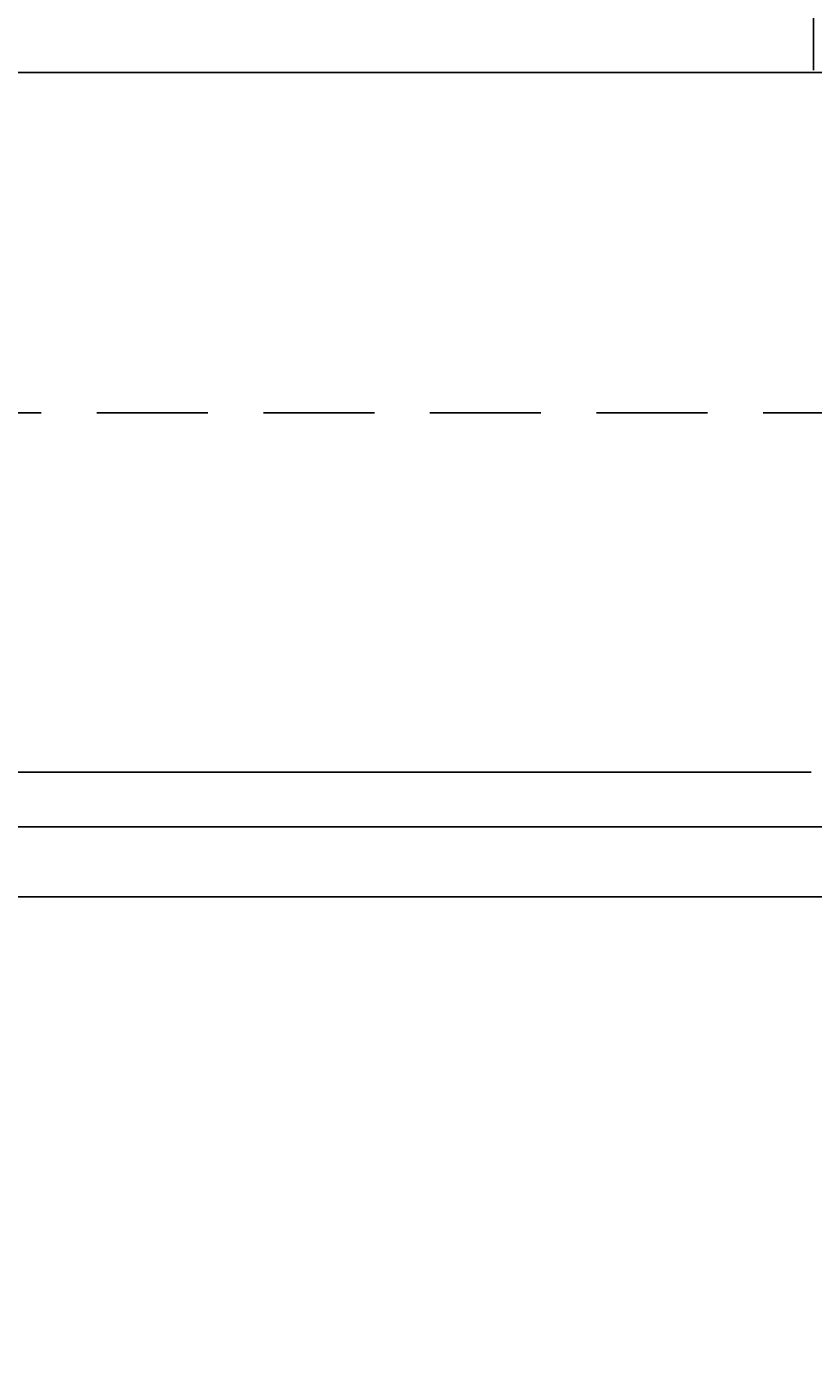
# Model space of a CAD drawing. Units: inches. Extents: x 2812 to 3051, y 1398 to 1659.
# Tile 6 of 65: x 2858 to 2880, y 1435 to 1473. Entities that reach past the tile are written whole.
import ezdxf

# ---------------------------------------------------------------- set-up
doc = ezdxf.new("R2010")
doc.units = ezdxf.units.IN
doc.linetypes.add('HIDDEN2', pattern=[4.7625, 3.175, -1.5875])
doc.layers.add('A-ANNO-DIMS', color=2, linetype='Continuous', lineweight=18)
doc.layers.add('S-CONC-HIDN', color=8, linetype='HIDDEN2', lineweight=25)
doc.styles.get("Standard").update_dxf_attribs({"font": 'arial.ttf'})
doc.dimstyles.get("Standard").update_dxf_attribs({"dimtxt": 0.18, "dimasz": 0.18, "dimexe": 0.18, "dimexo": 0.0625, "dimgap": 0.09, "dimtad": 0, "dimtih": 1, "dimtoh": 1, "dimdec": 4, "dimzin": 0, "dimdsep": 46, "dimtxsty": 'Standard', "dimcen": 0.09, "dimadec": 0, "dimazin": 0, "dimtfac": 1, "dimtdec": 4, "dimtofl": 0, "dimtmove": 0, "dimatfit": 3, "dimfxl": 1, "dimtolj": 1, "dimtzin": 0, "dimarcsym": 0})

# ---------------------------------------------------------------- blocks, each defined once
blk = doc.blocks.new('*D44')
at = {"layer": 'A-ANNO-DIMS', "color": 0, "lineweight": -2, "transparency": 16777216}
for p, q in [((2850.748, 1487.973), (2850.748, 1397.505)), ((2896.385, 1487.973), (2896.385, 1397.505)), ((2850.928, 1397.685), (2873.17, 1397.685)), ((2896.205, 1397.685), (2873.964, 1397.685))]:
    blk.add_line(p, q, dxfattribs=at)
at = {"layer": 'A-ANNO-DIMS', "color": 0, "transparency": 16777216}
for points in [[(2850.928, 1397.715), (2850.928, 1397.655), (2850.748, 1397.685)], [(2896.205, 1397.715), (2896.205, 1397.655), (2896.385, 1397.685)]]:
    blk.add_solid(points, dxfattribs=at)
at = {"layer": 'Defpoints', "color": 0, "transparency": 16777216}
for p in [(2850.748, 1488.035), (2896.385, 1488.035), (2896.385, 1397.685)]:
    blk.add_point(p, dxfattribs=at)
at = {"layer": 'A-ANNO-DIMS', "color": 0, "transparency": 16777216, "insert": (2873.567, 1397.685), "char_height": 0.18, "attachment_point": 5}
blk.add_mtext('\\A1;45.64', dxfattribs=at)
blk = doc.blocks.new('*D56')
at = {"layer": 'A-ANNO-DIMS', "color": 0, "lineweight": -2, "transparency": 16777216}
for p, q in [((2880.322, 1452.035), (2811.806, 1452.035)), ((2811.986, 1451.855), (2811.986, 1434.217)), ((2811.986, 1416.215), (2811.986, 1433.853)), ((2952.322, 1416.035), (2811.806, 1416.035))]:
    blk.add_line(p, q, dxfattribs=at)
at = {"layer": 'A-ANNO-DIMS', "color": 0, "transparency": 16777216}
for points in [[(2811.956, 1451.855), (2812.016, 1451.855), (2811.986, 1452.035)], [(2811.956, 1416.215), (2812.016, 1416.215), (2811.986, 1416.035)]]:
    blk.add_solid(points, dxfattribs=at)
at = {"layer": 'Defpoints', "color": 0, "transparency": 16777216}
for p in [(2811.986, 1452.035), (2880.385, 1452.035), (2952.385, 1416.035)]:
    blk.add_point(p, dxfattribs=at)
at = {"layer": 'A-ANNO-DIMS', "color": 0, "transparency": 16777216, "insert": (2811.986, 1434.035), "char_height": 0.18, "attachment_point": 5}
blk.add_mtext('\\A1;36', dxfattribs=at)
blk = doc.blocks.new('*D57')
at = {"layer": 'A-ANNO-DIMS', "color": 0, "lineweight": -2, "transparency": 16777216}
for p, q in [((2880.322, 1472.035), (2811.806, 1472.035)), ((2811.986, 1471.855), (2811.986, 1462.217)), ((2811.986, 1452.215), (2811.986, 1461.853)), ((2880.322, 1452.035), (2811.806, 1452.035))]:
    blk.add_line(p, q, dxfattribs=at)
at = {"layer": 'A-ANNO-DIMS', "color": 0, "transparency": 16777216}
for points in [[(2811.956, 1471.855), (2812.016, 1471.855), (2811.986, 1472.035)], [(2811.956, 1452.215), (2812.016, 1452.215), (2811.986, 1452.035)]]:
    blk.add_solid(points, dxfattribs=at)
at = {"layer": 'Defpoints', "color": 0, "transparency": 16777216}
for p in [(2811.986, 1472.035), (2880.385, 1472.035), (2880.385, 1452.035)]:
    blk.add_point(p, dxfattribs=at)
at = {"layer": 'A-ANNO-DIMS', "color": 0, "transparency": 16777216, "insert": (2811.986, 1462.035), "char_height": 0.18, "attachment_point": 5}
blk.add_mtext('\\A1;20', dxfattribs=at)
blk = doc.blocks.new('*D58')
at = {"layer": 'A-ANNO-DIMS', "color": 0, "lineweight": -2, "transparency": 16777216}
for p, q in [((2880.385, 1472.098), (2880.385, 1659.35)), ((2880.565, 1659.17), (2881.736, 1659.17)), ((2883.205, 1659.17), (2882.034, 1659.17)), ((2883.385, 1472.098), (2883.385, 1659.35))]:
    blk.add_line(p, q, dxfattribs=at)
at = {"layer": 'A-ANNO-DIMS', "color": 0, "transparency": 16777216}
for points in [[(2880.565, 1659.2), (2880.565, 1659.14), (2880.385, 1659.17)], [(2883.205, 1659.2), (2883.205, 1659.14), (2883.385, 1659.17)]]:
    blk.add_solid(points, dxfattribs=at)
at = {"layer": 'Defpoints', "color": 0, "transparency": 16777216}
for p in [(2883.385, 1659.17), (2880.385, 1472.035), (2883.385, 1472.035)]:
    blk.add_point(p, dxfattribs=at)
at = {"layer": 'A-ANNO-DIMS', "color": 0, "transparency": 16777216, "insert": (2881.885, 1659.17), "char_height": 0.18, "attachment_point": 5}
blk.add_mtext('\\A1;3', dxfattribs=at)
blk = doc.blocks.new('*D75')
at = {"layer": 'A-ANNO-DIMS', "color": 0, "lineweight": -2, "transparency": 16777216}
for p, q in [((2963.812, 1448.474), (2811.806, 1448.474)), ((2811.986, 1448.294), (2811.986, 1432.437)), ((2811.986, 1416.215), (2811.986, 1432.073)), ((2961.322, 1416.035), (2811.806, 1416.035))]:
    blk.add_line(p, q, dxfattribs=at)
at = {"layer": 'A-ANNO-DIMS', "color": 0, "transparency": 16777216}
for points in [[(2811.956, 1448.294), (2812.016, 1448.294), (2811.986, 1448.474)], [(2811.956, 1416.215), (2812.016, 1416.215), (2811.986, 1416.035)]]:
    blk.add_solid(points, dxfattribs=at)
at = {"layer": 'Defpoints', "color": 0, "transparency": 16777216}
for p in [(2811.986, 1448.474), (2963.874, 1448.474), (2961.385, 1416.035)]:
    blk.add_point(p, dxfattribs=at)
at = {"layer": 'A-ANNO-DIMS', "color": 0, "transparency": 16777216, "insert": (2811.986, 1432.255), "char_height": 0.18, "attachment_point": 5}
blk.add_mtext('\\A1;32.44', dxfattribs=at)
blk = doc.blocks.new('*D76')
at = {"layer": 'A-ANNO-DIMS', "color": 0, "lineweight": -2, "transparency": 16777216}
for p, q in [((2963.812, 1450.474), (2811.806, 1450.474)), ((2811.986, 1450.294), (2811.986, 1449.654)), ((2811.986, 1448.654), (2811.986, 1449.293)), ((2963.812, 1448.474), (2811.806, 1448.474))]:
    blk.add_line(p, q, dxfattribs=at)
at = {"layer": 'A-ANNO-DIMS', "color": 0, "transparency": 16777216}
for points in [[(2811.956, 1450.294), (2812.016, 1450.294), (2811.986, 1450.474)], [(2811.956, 1448.654), (2812.016, 1448.654), (2811.986, 1448.474)]]:
    blk.add_solid(points, dxfattribs=at)
at = {"layer": 'Defpoints', "color": 0, "transparency": 16777216}
for p in [(2811.986, 1450.474), (2963.874, 1450.474), (2963.874, 1448.474)]:
    blk.add_point(p, dxfattribs=at)
at = {"layer": 'A-ANNO-DIMS', "color": 0, "transparency": 16777216, "insert": (2811.986, 1449.474), "char_height": 0.18, "attachment_point": 5}
blk.add_mtext('\\A1;2', dxfattribs=at)
blk = doc.blocks.new('*D77')
at = {"layer": 'A-ANNO-DIMS', "color": 0, "lineweight": -2, "transparency": 16777216}
for p, q in [((2961.322, 1472.035), (2811.806, 1472.035)), ((2811.986, 1471.855), (2811.986, 1461.436)), ((2811.986, 1450.654), (2811.986, 1461.073)), ((2963.812, 1450.474), (2811.806, 1450.474))]:
    blk.add_line(p, q, dxfattribs=at)
at = {"layer": 'A-ANNO-DIMS', "color": 0, "transparency": 16777216}
for points in [[(2811.956, 1471.855), (2812.016, 1471.855), (2811.986, 1472.035)], [(2811.956, 1450.654), (2812.016, 1450.654), (2811.986, 1450.474)]]:
    blk.add_solid(points, dxfattribs=at)
at = {"layer": 'Defpoints', "color": 0, "transparency": 16777216}
for p in [(2811.986, 1472.035), (2961.385, 1472.035), (2963.874, 1450.474)]:
    blk.add_point(p, dxfattribs=at)
at = {"layer": 'A-ANNO-DIMS', "color": 0, "transparency": 16777216, "insert": (2811.986, 1461.255), "char_height": 0.18, "attachment_point": 5}
blk.add_mtext('\\A1;21.56', dxfattribs=at)

msp = doc.modelspace()

# ---------------------------------------------------------------- linework, layer by layer
at = {"layer": 'S-CONC-HIDN'}
msp.add_line((3029.7562, 1462.3026), (2835.3849, 1462.3026), dxfattribs=at)

# ---------------------------------------------------------------- dimensions: what is measured, and where the dimension line sits
at = {"layer": 'A-ANNO-DIMS'}
for base, p1, p2, override, picture, middle in [((2883.3849, 1659.17), (2880.3849, 1472.0354), (2883.3849, 1472.0354), {"dimdec": 0, "dimlfac": 1, "dimrnd": 0, "dimzin": 0, "dimdsep": 46, "dimlunit": 2}, '*D58', (2881.8849, 1659.17)), ((2896.3849, 1397.6854), (2850.7485, 1488.0354), (2896.3849, 1488.0354), {"dimdec": 2, "dimlfac": 1, "dimrnd": 0, "dimzin": 0, "dimdsep": 46, "dimlunit": 2}, '*D44', (2873.5667, 1397.6854))]:
    dim = msp.add_linear_dim(base=base, p1=p1, p2=p2, dimstyle='Standard', override=override, dxfattribs=at)
    dim.commit()
    dim.dimension.update_dxf_attribs({"geometry": picture, "text_midpoint": middle})
for base, p1, p2, override, picture, middle in [((2811.9855, 1472.0354), (2963.8741, 1450.4738), (2961.3849, 1472.0354), {"dimdec": 2, "dimlfac": 1, "dimrnd": 0, "dimzin": 0, "dimdsep": 46, "dimlunit": 2}, '*D77', (2811.9855, 1461.2546)), ((2811.9855, 1472.0354), (2880.3849, 1452.0354), (2880.3849, 1472.0354), {"dimdec": 0, "dimlfac": 1, "dimrnd": 0, "dimzin": 0, "dimdsep": 46, "dimlunit": 2}, '*D57', (2811.9855, 1462.0354)), ((2811.9855, 1452.0354), (2952.3849, 1416.0354), (2880.3849, 1452.0354), {"dimdec": 0, "dimlfac": 1, "dimrnd": 0, "dimzin": 0, "dimdsep": 46, "dimlunit": 2}, '*D56', (2811.9855, 1434.0354)), ((2811.9855, 1450.4738), (2963.8741, 1448.4738), (2963.8741, 1450.4738), {"dimdec": 0, "dimlfac": 1, "dimrnd": 0, "dimzin": 0, "dimdsep": 46, "dimlunit": 2}, '*D76', (2811.9855, 1449.4738)), ((2811.9855, 1448.4738), (2961.3849, 1416.0354), (2963.8741, 1448.4738), {"dimdec": 2, "dimlfac": 1, "dimrnd": 0, "dimzin": 0, "dimdsep": 46, "dimlunit": 2}, '*D75', (2811.9855, 1432.2546))]:
    dim = msp.add_linear_dim(base=base, p1=p1, p2=p2, angle=90, dimstyle='Standard', override=override, dxfattribs=at)
    dim.commit()
    dim.dimension.update_dxf_attribs({"geometry": picture, "text_midpoint": middle})

doc.saveas('drawing.dxf')
